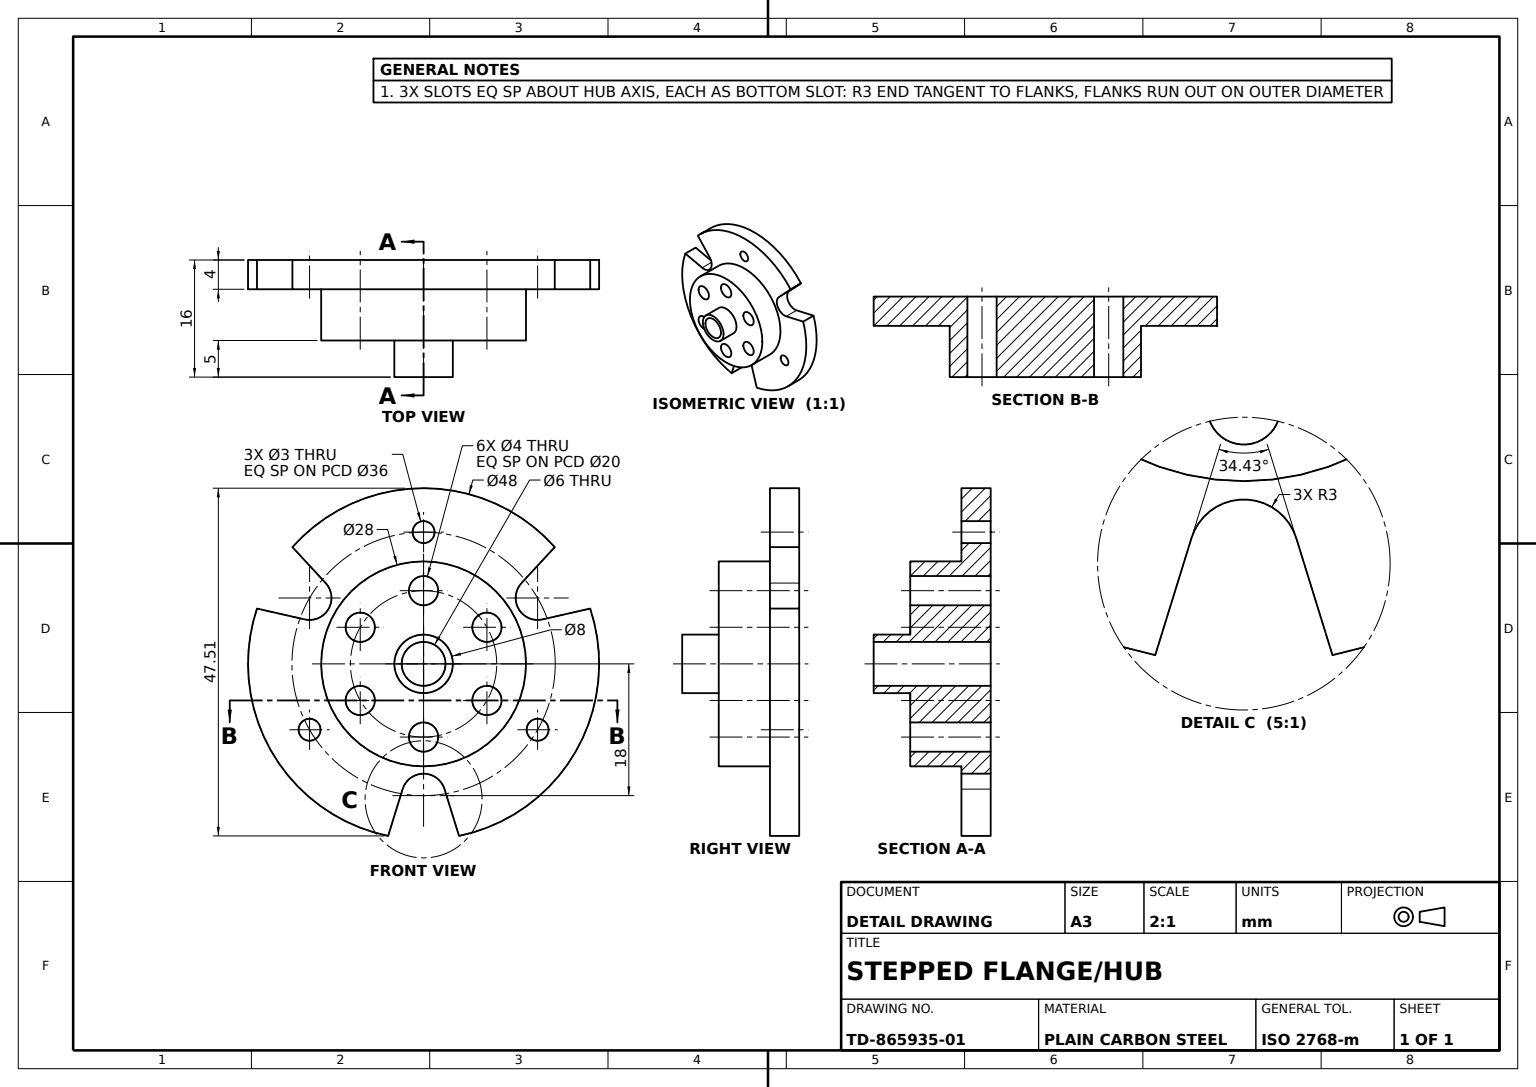
SolidWorks part; units mm, degrees
material "Plain Carbon Steel"
ref_plane "Front Plane" through (0, 0, 0) normal (0, 0, 1) x (1, 0, 0)
ref_plane "Top Plane" through (0, 0, 0) normal (0, 1, 0) x (1, 0, 0)
ref_plane "Right Plane" through (0, 0, 0) normal (1, 0, 0) x (0, 0, -1)
sketch "Flange Profile Sketch" plane through (0, 0, 0) normal (0, 0, 1) x (1, 0, 0)
  line L0 (0, 0) -> (24, 0) construction
  line L1 (0, 0) -> (0, 24) construction
  line L2 (0, 0) -> (-24, 0) construction
  line L3 (0, 0) -> (0, -24) construction
  line L5 (4.8468, -23.5055) -> (2.8656, -17.112)
  line L7 (-4.8468, -23.5055) -> (-2.8656, -17.112)
  line L8 (-22.7797, 7.5553) -> (-16.2522, 6.0744)
  line L9 (17.933, 15.9502) -> (13.3867, 11.0377)
  line L10 (-17.933, 15.9502) -> (-13.3867, 11.0377)
  line L11 (22.7797, 7.5553) -> (16.2522, 6.0744)
  arc A0 (4.8468, -23.5055) -> (22.7797, 7.5553) centre (0, 0) ccw
  circle A1 centre (0, 0) radius 18 construction
  arc A2 (2.8656, -17.112) -> (-2.8656, -17.112) centre (0, -18) ccw
  arc A3 (-16.2522, 6.0744) -> (-13.3867, 11.0377) centre (-15.5885, 9) ccw
  arc A4 (13.3867, 11.0377) -> (16.2522, 6.0744) centre (15.5885, 9) ccw
  arc A5 (-22.7797, 7.5553) -> (-4.8468, -23.5055) centre (0, 0) ccw
  arc A6 (17.933, 15.9502) -> (-17.933, 15.9502) centre (0, 0) ccw
  dimension "D1" = 48
  dimension "D2" = 36
  dimension "D3" = 3
  dimension "D4" = 4.8468
  dimension "D5" = 6.888
  dimension "D6" = 2.8656
  dimension "D7" = 3
  dimension "D8" = 3
  dimension "D9" = 3
extrude "Slotted Flange Ø48" add sketch "Flange Profile Sketch" along normal blind 4
sketch "Hub Sketch" plane through (0, 0, 4) normal (0, 0, 1) x (1, 0, 0)
  circle A0 centre (0, 0) radius 14
  dimension "D1" = 28
extrude "Hub Ø28" add sketch "Hub Sketch" along normal blind 7
sketch "Hub Holes Sketch" plane through (0, 0, 11) normal (0, 0, 1) x (1, 0, 0)
  line L0 (0, 0) -> (0, 10)
  circle A0 centre (0, 0) radius 10
  circle A1 centre (0, 10) radius 2
  circle A2 centre (8.6603, 5) radius 2
  circle A3 centre (8.6603, -5) radius 2
  circle A4 centre (0, -10) radius 2
  circle A5 centre (-8.6603, -5) radius 2
  circle A6 centre (-8.6603, 5) radius 2
  dimension "D1" = 20
  dimension "D2" = 4
  dimension "D3" = 8.6603
  dimension "D4" = 10
extrude "Hub Holes 6xØ4" cut sketch "Hub Holes Sketch" against normal blind 30 contours A0 A6 | A0 A6 | A0 A5 | A0 A5 | A0 A4 | A0 A4 | A0 A3 | A0 A3 | A0 A2 | A0 A2 | A0 A1 | L0 A1 A0 | A0 A1 L0
sketch "Spigot Sketch" plane through (0, 0, 11) normal (0, 0, 1) x (1, 0, 0)
  circle A0 centre (0, 0) radius 4
  dimension "D1" = 8
extrude "Spigot Ø8" add sketch "Spigot Sketch" along normal blind 5
sketch "Bore Sketch" plane through (0, 0, 16) normal (0, 0, 1) x (1, 0, 0)
  circle A0 centre (0, 0) radius 3
  dimension "D1" = 6
extrude "Bore Ø6" cut sketch "Bore Sketch" against normal blind 50
sketch "Flange Holes Sketch" plane through (0, 0, 4) normal (0, 0, 1) x (1, 0, 0)
  line L0 (0, 0) -> (0, 18)
  circle A0 centre (15.5885, -9) radius 1.5
  circle A1 centre (0, 0) radius 18
  circle A2 centre (0, 18) radius 1.5
  circle A3 centre (-15.5885, -9) radius 1.5
  dimension "D1" = 36
  dimension "D2" = 3
  dimension "D4" = 31.1769
  dimension "D5" = 27
  dimension "D3" = 3
extrude "Flange Holes 3xØ3" cut sketch "Flange Holes Sketch" against normal blind 30 contours A1 A2 L0 | L0 A2 A1 | A1 A2 | A1 A3 | A1 A3 | A1 A0 | A0 A1
